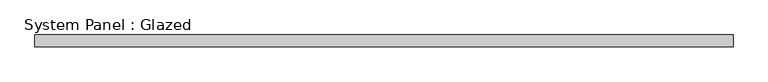
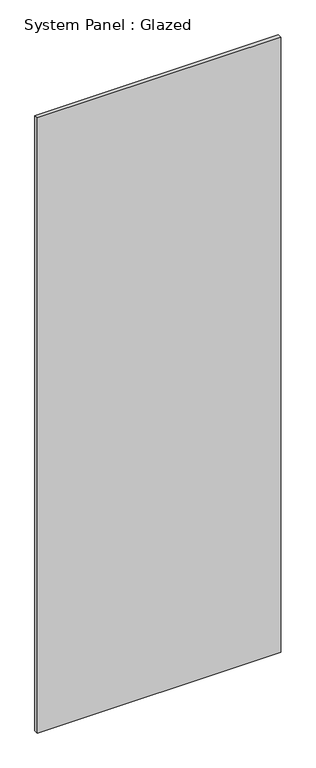
"""IFC4 building model written with IfcOpenShell, lengths in millimetres: plate geometry, System Panel : Glazed."""

from ifc_helpers import new_model, si_unit, origin, origin_with_axes, place, context, project, spatial, polyline, outline, extrude, source, transform, mapped, element, save


def system_panel_glazed_6806f88e(model_context):
    return source(origin(), model_context, "Body", "SweptSolid", [
        extrude(outline(polyline([(748.9304629, 24.5), (-748.9304629, 24.5), (-748.9304629, 49.5), (748.9304629, 49.5), (748.9304629, 24.5)])), origin_with_axes(), (0.0, 0.0, 1.0), 4000.0),
    ])


if __name__ == "__main__":
    model = new_model("IFC4")
    model_context = context("Model", 3, world=origin())
    ifc_project = project(units=[si_unit("LENGTHUNIT", "METRE", prefix="MILLI")], contexts=[model_context])
    site = spatial("IfcSite", under=ifc_project)
    building = spatial("IfcBuilding", under=site)
    placement = place(None, origin())
    system_panel_glazed_shape = system_panel_glazed_6806f88e(model_context)
    element("IfcPlate", 1, ObjectType="System Panel : Glazed", at=placement, inside=building, context=model_context, shape_type="MappedRepresentation", body=[
        mapped(system_panel_glazed_shape, transform((0.0, 0.0, 0.0), x_axis=(1.0, 0.0, 0.0), y_axis=(0.0, 1.0, 0.0), z_axis=(0.0, 0.0, 1.0))),
    ])
    save(model, "model.ifc")

# Revit data of these elements
# Type "System Panel : Glazed"
#   Keynote = "H11"
#   Construction Type Id = "GSP4R"
#   Analytic Construction = "1/8 in Pilkington single glazing"
#   Visual Light Transmittance = 0.9
#   Solar Heat Gain Coefficient = 0.86
#   Heat Transfer Coefficient (U) = 6.7069 W/(m²·K)
#   Define Thermal Properties by = 1
# Element 1 (IfcPlate, "System Panel : Glazed")
#   Materials on its faces: "Glass"
# Materials
#   "Glass": class "Glass", colour RGB 0 128 192, transparency 0.9, Description = "Soda Lime Glass", Cost = 0
